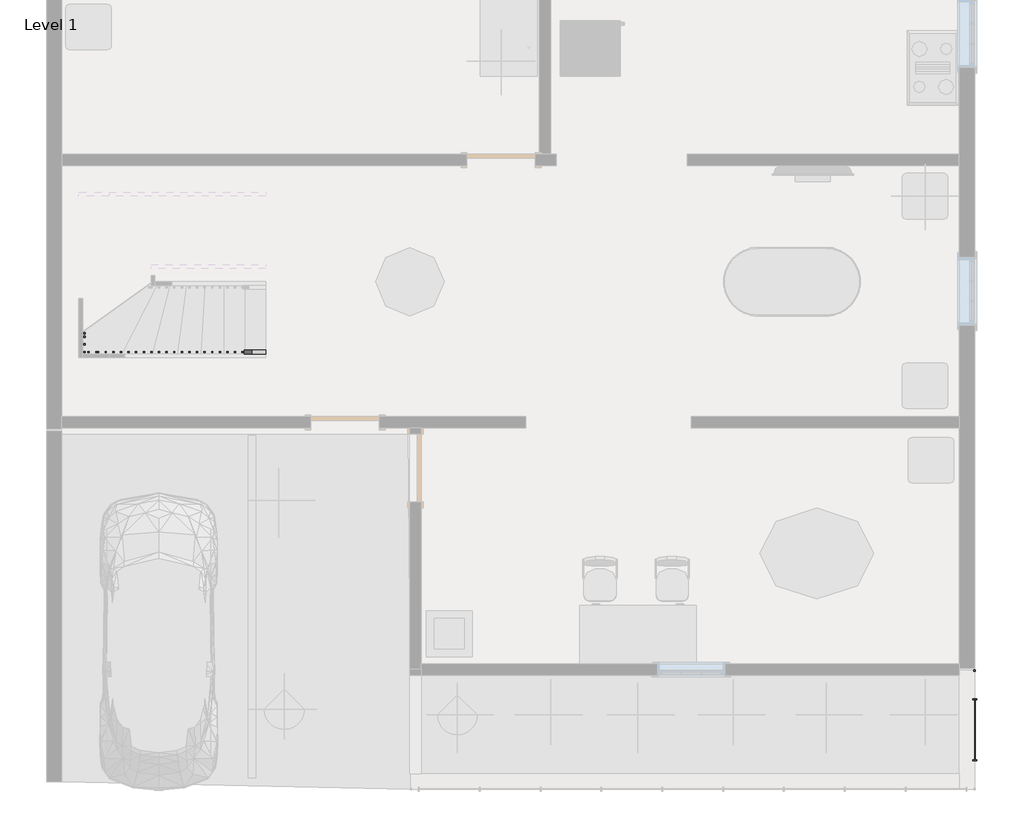
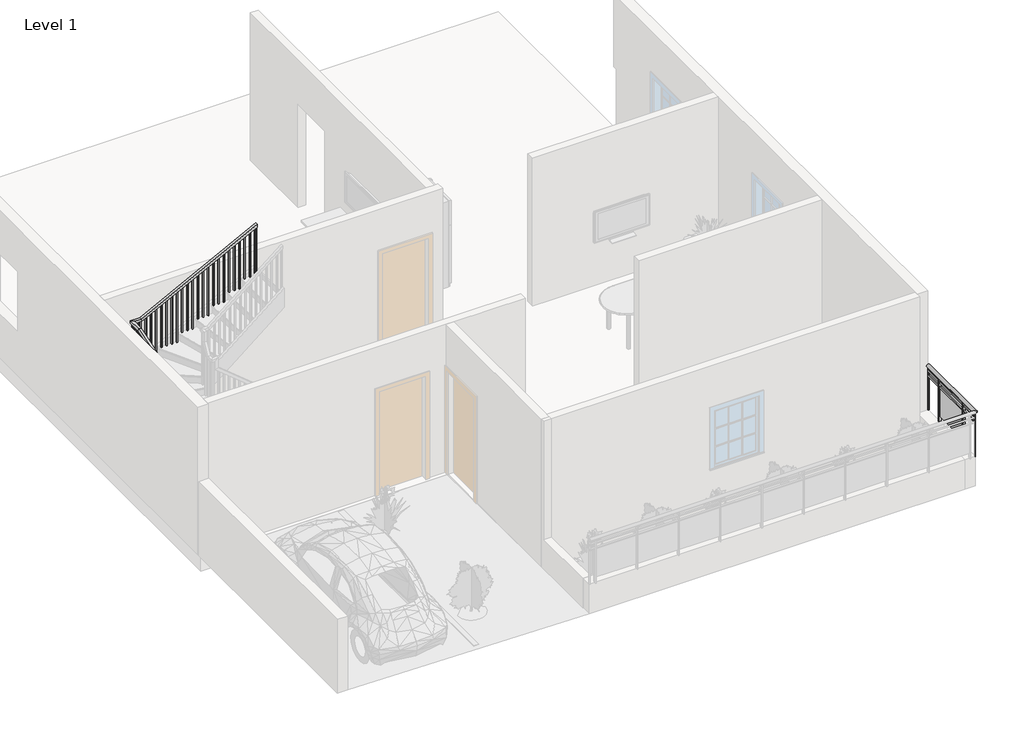
# One storey, part 2 of 3: 2 railings.
"""IFC4 building model written with IfcOpenShell, lengths in millimetres."""

from ifc_helpers import new_model, si_unit, point, frame, origin, place, context, project, spatial, polyline, ellipse_curve, trimmed, outline, extrude, faceted_brep, element, save
from ifc_brep_helpers import plane_surface, extruded_surface, advanced_brep

model = new_model("IFC4")

# Units and contexts
model_context = context("Model", 3, world=origin())
ifc_project = project(units=[si_unit("LENGTHUNIT", "METRE", prefix="MILLI")], contexts=[model_context])

# Site, building, storey
site = spatial("IfcSite", under=ifc_project)
building = spatial("IfcBuilding", under=site)
storey = spatial("IfcBuildingStorey", under=building, Name="Level 1", Elevation=0.0)

# Railings
placement = place(None, origin())
element("IfcRailing", 1, ObjectType="Glass Panel - Bottom Fill", at=placement, inside=storey, context=model_context, shape_type="SolidModel", body=[
    advanced_brep(
    [(-291.5234692, -2386.0883114, 1524.0), (-367.7234692, -2386.0883114, 1524.0), (-291.5234692, -3973.5883114, 1524.0), (-367.7234692, -3973.5883114, 1524.0)],
    [
        (0, 1, ellipse_curve(frame((-329.6234692, -2386.0883114, 1524.0), z_axis=(0.0, 1.0, 0.0), x_axis=(-1.0, 0.0, 0.0)), 38.1, 28.575)),
        (1, 0, ellipse_curve(frame((-329.6234692, -2386.0883114, 1524.0), z_axis=(0.0, 1.0, 0.0), x_axis=(-1.0, 0.0, 0.0)), 38.1, 28.575)),
        (2, 3, ellipse_curve(frame((-329.6234692, -3973.5883114, 1524.0), z_axis=(0.0, -1.0, 0.0), x_axis=(-1.0, 0.0, 0.0)), 38.1, 28.575)),
        (3, 2, ellipse_curve(frame((-329.6234692, -3973.5883114, 1524.0), z_axis=(0.0, -1.0, 0.0), x_axis=(-1.0, 0.0, 0.0)), 38.1, 28.575)),
        (0, 2),
        (3, 1),
    ],
    [
        plane_surface(frame((-329.6234692, -2386.0883114, 1524.0), z_axis=(0.0, 1.0, 0.0), x_axis=(0.0, 0.0, -1.0))),
        plane_surface(frame((-329.6234692, -3973.5883114, 1524.0), z_axis=(0.0, -1.0, 0.0), x_axis=(0.0, 0.0, -1.0))),
        extruded_surface(trimmed(ellipse_curve(frame((-329.6234692, -3973.5883114, 1524.0), z_axis=(0.0, 1.0, 0.0), x_axis=(-1.0, 0.0, 0.0)), 38.1, 28.575), [point((-291.5234692, -3973.5883114, 1524.0))], [point((-367.7234692, -3973.5883114, 1524.0))], True, "CARTESIAN"), (0.0, 1587.5, 0.0), 1587.5),
        extruded_surface(trimmed(ellipse_curve(frame((-329.6234692, -3973.5883114, 1524.0), z_axis=(0.0, 1.0, 0.0), x_axis=(-1.0, 0.0, 0.0)), 38.1, 28.575), [point((-367.7234692, -3973.5883114, 1524.0))], [point((-291.5234692, -3973.5883114, 1524.0))], True, "CARTESIAN"), (0.0, 1587.5, 0.0), 1587.5),
    ],
    [
        (0, [[1, 2]]),
        (1, [[3, 4]]),
        (2, [[-1, 5, -4, 6]]),
        (3, [[-2, -6, -3, -5]]),
    ],
),
    extrude(outline(polyline([(-342.3234692, -2386.0883114), (-316.9234692, -2386.0883114), (-316.9234692, -3973.5883114), (-342.3234692, -3973.5883114), (-342.3234692, -2386.0883114)])), frame((0.0, 0.0, 1409.7), z_axis=(0.0, 0.0, 1.0), x_axis=(1.0, 0.0, 0.0)), (0.0, 0.0, 1.0), 25.4),
    extrude(outline(polyline([(-342.3234692, -2386.0883114), (-316.9234692, -2386.0883114), (-316.9234692, -3973.5883114), (-342.3234692, -3973.5883114), (-342.3234692, -2386.0883114)])), frame((0.0, 0.0, 1308.1), z_axis=(0.0, 0.0, 1.0), x_axis=(1.0, 0.0, 0.0)), (0.0, 0.0, 1.0), 25.4),
    extrude(outline(polyline([(-355.0234692, -3579.8883114), (-304.2234692, -3579.8883114), (-304.2234692, -3592.5883114), (-355.0234692, -3592.5883114), (-355.0234692, -3579.8883114)])), frame((0.0, 0.0, 609.6), z_axis=(0.0, 0.0, 1.0), x_axis=(1.0, 0.0, 0.0)), (0.0, 0.0, 1.0), 885.6788223),
    extrude(outline(polyline([(-323.0883121, -2773.4383114), (-323.0883121, -3586.2383114), (-329.4383121, -3586.2383114), (-329.4383121, -2773.4383114), (-323.0883121, -2773.4383114)])), frame((0.0, 0.0, 711.2), z_axis=(0.0, 0.0, 1.0), x_axis=(1.0, 0.0, 0.0)), (0.0, 0.0, 1.0), 596.9),
    extrude(outline(polyline([(-355.0234692, -2767.0883114), (-304.2234692, -2767.0883114), (-304.2234692, -2779.7883114), (-355.0234692, -2779.7883114), (-355.0234692, -2767.0883114)])), frame((0.0, 0.0, 609.6), z_axis=(0.0, 0.0, 1.0), x_axis=(1.0, 0.0, 0.0)), (0.0, 0.0, 1.0), 885.6788223),
    extrude(outline(polyline([(-339.1484692, -3960.8883114), (-320.0984692, -3960.8883114), (-320.0984692, -3979.9383114), (-339.1484692, -3979.9383114), (-339.1484692, -3960.8883114)])), frame((0.0, 0.0, 609.6), z_axis=(0.0, 0.0, 1.0), x_axis=(1.0, 0.0, 0.0)), (0.0, 0.0, 1.0), 885.6788223),
    extrude(outline(polyline([(-339.1484692, -2379.7383114), (-320.0984692, -2379.7383114), (-320.0984692, -2398.7883114), (-339.1484692, -2398.7883114), (-339.1484692, -2379.7383114)])), frame((0.0, 0.0, 609.6), z_axis=(0.0, 0.0, 1.0), x_axis=(1.0, 0.0, 0.0)), (0.0, 0.0, 1.0), 885.6788223),
])
element("IfcRailing", 2, ObjectType="Handrail - Rectangular", at=placement, inside=storey, context=model_context, shape_type="SolidModel", body=[
    faceted_brep([(-9800.0917773, 1843.0116886, 1109.0771751), (-9800.0917773, 1843.0116886, 1051.9280057), (-9800.0917773, 1893.8116886, 1051.9280057), (-9800.0917773, 1893.8116886, 1109.0771751), (-12060.0736338, 1843.0116886, 2273.7644996), (-12072.3936851, 1843.0116886, 2222.9644996), (-12072.3936851, 1893.8116886, 2222.9644996), (-12060.0736338, 1893.8116886, 2273.7644996), (-12242.2234692, 1843.0116886, 2273.7644996), (-12242.2234692, 1843.0116886, 2222.9644996), (-12191.4234692, 1893.8116886, 2222.9644996), (-12191.4234692, 1893.8116886, 2273.7644996), (-12242.2234692, 2120.1656412, 2273.7644996), (-12242.2234692, 2128.1162174, 2222.9644996), (-12191.4234692, 2128.1162174, 2222.9644996), (-12191.4234692, 2120.1656412, 2273.7644996), (-12242.2234692, 3674.057736, 2772.3688337), (-12242.2234692, 3682.0083121, 2721.5688337), (-12191.4234692, 3682.0083121, 2721.5688337), (-12191.4234692, 3674.057736, 2772.3688337), (-12242.2234692, 3951.2116886, 2772.3688337), (-12242.2234692, 3951.2116886, 2721.5688337), (-12191.4234692, 3900.4116886, 2721.5688337), (-12191.4234692, 3900.4116886, 2772.3688337), (-12060.0736338, 3951.2116886, 2772.3688337), (-12047.7535825, 3951.2116886, 2721.5688337), (-12047.7535825, 3900.4116886, 2721.5688337), (-12060.0736338, 3900.4116886, 2772.3688337), (-9800.0917773, 3951.2116886, 3937.0561582), (-9800.0917773, 3900.4116886, 3937.0561582), (-9800.0917773, 3900.4116886, 3879.9069889), (-9800.0917773, 3951.2116886, 3879.9069889)], [[[0, 1, 2, 3]], [[1, 0, 4, 5]], [[2, 1, 5, 6]], [[3, 2, 6, 7]], [[0, 3, 7, 4]], [[5, 4, 8, 9]], [[6, 5, 9, 10]], [[7, 6, 10, 11]], [[4, 7, 11, 8]], [[9, 8, 12, 13]], [[10, 9, 13, 14]], [[11, 10, 14, 15]], [[8, 11, 15, 12]], [[13, 12, 16, 17]], [[14, 13, 17, 18]], [[15, 14, 18, 19]], [[12, 15, 19, 16]], [[17, 16, 20, 21]], [[18, 17, 21, 22]], [[19, 18, 22, 23]], [[16, 19, 23, 20]], [[21, 20, 24, 25]], [[22, 21, 25, 26]], [[23, 22, 26, 27]], [[20, 23, 27, 24]], [[28, 29, 30, 31]], [[25, 24, 28, 31]], [[26, 25, 31, 30]], [[27, 26, 30, 29]], [[24, 27, 29, 28]]]),
    extrude(outline(polyline([(3862.2268642, -9834.3986338), (2878.6666667, -9834.3986338), (2878.6666667, -9815.3486338), (3872.0443296, -9815.3486338), (3862.2268642, -9834.3986338)])), frame((0.0, 3916.2866886, 0.0), z_axis=(0.0, 1.0, 0.0), x_axis=(0.0, 0.0, 1.0)), (0.0, 0.0, 1.0), 19.05),
    extrude(outline(polyline([(3809.8670491, -9935.9986338), (2878.6666667, -9935.9986338), (2878.6666667, -9916.9486338), (3819.6845145, -9916.9486338), (3809.8670491, -9935.9986338)])), frame((0.0, 3916.2866886, 0.0), z_axis=(0.0, 1.0, 0.0), x_axis=(0.0, 0.0, 1.0)), (0.0, 0.0, 1.0), 19.05),
    extrude(outline(polyline([(3757.507234, -10037.5986338), (2878.6666667, -10037.5986338), (2878.6666667, -10018.5486338), (3767.3246993, -10018.5486338), (3757.507234, -10037.5986338)])), frame((0.0, 3916.2866886, 0.0), z_axis=(0.0, 1.0, 0.0), x_axis=(0.0, 0.0, 1.0)), (0.0, 0.0, 1.0), 19.05),
    extrude(outline(polyline([(3705.1474189, -10139.1986338), (2709.3333333, -10139.1986338), (2709.3333333, -10120.1486338), (3714.9648842, -10120.1486338), (3705.1474189, -10139.1986338)])), frame((0.0, 3916.2866886, 0.0), z_axis=(0.0, 1.0, 0.0), x_axis=(0.0, 0.0, 1.0)), (0.0, 0.0, 1.0), 19.05),
    extrude(outline(polyline([(3652.7876038, -10240.7986338), (2709.3333333, -10240.7986338), (2709.3333333, -10221.7486338), (3662.6050691, -10221.7486338), (3652.7876038, -10240.7986338)])), frame((0.0, 3916.2866886, 0.0), z_axis=(0.0, 1.0, 0.0), x_axis=(0.0, 0.0, 1.0)), (0.0, 0.0, 1.0), 19.05),
    extrude(outline(polyline([(3600.4277887, -10342.3986338), (2709.3333333, -10342.3986338), (2709.3333333, -10323.3486338), (3610.245254, -10323.3486338), (3600.4277887, -10342.3986338)])), frame((0.0, 3916.2866886, 0.0), z_axis=(0.0, 1.0, 0.0), x_axis=(0.0, 0.0, 1.0)), (0.0, 0.0, 1.0), 19.05),
    extrude(outline(polyline([(3548.0679735, -10443.9986338), (2540.0, -10443.9986338), (2540.0, -10424.9486338), (3557.8854389, -10424.9486338), (3548.0679735, -10443.9986338)])), frame((0.0, 3916.2866886, 0.0), z_axis=(0.0, 1.0, 0.0), x_axis=(0.0, 0.0, 1.0)), (0.0, 0.0, 1.0), 19.05),
    extrude(outline(polyline([(3495.7081584, -10545.5986338), (2540.0, -10545.5986338), (2540.0, -10526.5486338), (3505.5256238, -10526.5486338), (3495.7081584, -10545.5986338)])), frame((0.0, 3916.2866886, 0.0), z_axis=(0.0, 1.0, 0.0), x_axis=(0.0, 0.0, 1.0)), (0.0, 0.0, 1.0), 19.05),
    extrude(outline(polyline([(3443.3483433, -10647.1986338), (2540.0, -10647.1986338), (2540.0, -10628.1486338), (3453.1658086, -10628.1486338), (3443.3483433, -10647.1986338)])), frame((0.0, 3916.2866886, 0.0), z_axis=(0.0, 1.0, 0.0), x_axis=(0.0, 0.0, 1.0)), (0.0, 0.0, 1.0), 19.05),
    extrude(outline(polyline([(3390.9885282, -10748.7986338), (2370.6666667, -10748.7986338), (2370.6666667, -10729.7486338), (3400.8059935, -10729.7486338), (3390.9885282, -10748.7986338)])), frame((0.0, 3916.2866886, 0.0), z_axis=(0.0, 1.0, 0.0), x_axis=(0.0, 0.0, 1.0)), (0.0, 0.0, 1.0), 19.05),
    extrude(outline(polyline([(3338.6287131, -10850.3986338), (2370.6666667, -10850.3986338), (2370.6666667, -10831.3486338), (3348.4461784, -10831.3486338), (3338.6287131, -10850.3986338)])), frame((0.0, 3916.2866886, 0.0), z_axis=(0.0, 1.0, 0.0), x_axis=(0.0, 0.0, 1.0)), (0.0, 0.0, 1.0), 19.05),
    extrude(outline(polyline([(3286.268898, -10951.9986338), (2370.6666667, -10951.9986338), (2370.6666667, -10932.9486338), (3296.0863633, -10932.9486338), (3286.268898, -10951.9986338)])), frame((0.0, 3916.2866886, 0.0), z_axis=(0.0, 1.0, 0.0), x_axis=(0.0, 0.0, 1.0)), (0.0, 0.0, 1.0), 19.05),
    extrude(outline(polyline([(3233.9090828, -11053.5986338), (2201.3333333, -11053.5986338), (2201.3333333, -11034.5486338), (3243.7265482, -11034.5486338), (3233.9090828, -11053.5986338)])), frame((0.0, 3916.2866886, 0.0), z_axis=(0.0, 1.0, 0.0), x_axis=(0.0, 0.0, 1.0)), (0.0, 0.0, 1.0), 19.05),
    extrude(outline(polyline([(3181.5492677, -11155.1986338), (2201.3333333, -11155.1986338), (2201.3333333, -11136.1486338), (3191.3667331, -11136.1486338), (3181.5492677, -11155.1986338)])), frame((0.0, 3916.2866886, 0.0), z_axis=(0.0, 1.0, 0.0), x_axis=(0.0, 0.0, 1.0)), (0.0, 0.0, 1.0), 19.05),
    extrude(outline(polyline([(3129.1894526, -11256.7986338), (2201.3333333, -11256.7986338), (2201.3333333, -11237.7486338), (3139.0069179, -11237.7486338), (3129.1894526, -11256.7986338)])), frame((0.0, 3916.2866886, 0.0), z_axis=(0.0, 1.0, 0.0), x_axis=(0.0, 0.0, 1.0)), (0.0, 0.0, 1.0), 19.05),
    extrude(outline(polyline([(3076.8296375, -11358.3986338), (2032.0, -11358.3986338), (2032.0, -11339.3486338), (3086.6471028, -11339.3486338), (3076.8296375, -11358.3986338)])), frame((0.0, 3916.2866886, 0.0), z_axis=(0.0, 1.0, 0.0), x_axis=(0.0, 0.0, 1.0)), (0.0, 0.0, 1.0), 19.05),
    extrude(outline(polyline([(3024.4698224, -11459.9986338), (2032.0, -11459.9986338), (2032.0, -11440.9486338), (3034.2872877, -11440.9486338), (3024.4698224, -11459.9986338)])), frame((0.0, 3916.2866886, 0.0), z_axis=(0.0, 1.0, 0.0), x_axis=(0.0, 0.0, 1.0)), (0.0, 0.0, 1.0), 19.05),
    extrude(outline(polyline([(2972.1100073, -11561.5986338), (2032.0, -11561.5986338), (2032.0, -11542.5486338), (2981.9274726, -11542.5486338), (2972.1100073, -11561.5986338)])), frame((0.0, 3916.2866886, 0.0), z_axis=(0.0, 1.0, 0.0), x_axis=(0.0, 0.0, 1.0)), (0.0, 0.0, 1.0), 19.05),
    extrude(outline(polyline([(2919.7501921, -11663.1986338), (2032.0, -11663.1986338), (2032.0, -11644.1486338), (2929.5676575, -11644.1486338), (2919.7501921, -11663.1986338)])), frame((0.0, 3916.2866886, 0.0), z_axis=(0.0, 1.0, 0.0), x_axis=(0.0, 0.0, 1.0)), (0.0, 0.0, 1.0), 19.05),
    extrude(outline(polyline([(2867.390377, -11764.7986338), (1862.6666667, -11764.7986338), (1862.6666667, -11745.7486338), (2877.2078424, -11745.7486338), (2867.390377, -11764.7986338)])), frame((0.0, 3916.2866886, 0.0), z_axis=(0.0, 1.0, 0.0), x_axis=(0.0, 0.0, 1.0)), (0.0, 0.0, 1.0), 19.05),
    extrude(outline(polyline([(2815.0305619, -11866.3986338), (1862.6666667, -11866.3986338), (1862.6666667, -11847.3486338), (2824.8480272, -11847.3486338), (2815.0305619, -11866.3986338)])), frame((0.0, 3916.2866886, 0.0), z_axis=(0.0, 1.0, 0.0), x_axis=(0.0, 0.0, 1.0)), (0.0, 0.0, 1.0), 19.05),
    extrude(outline(polyline([(2762.6707468, -11967.9986338), (1862.6666667, -11967.9986338), (1862.6666667, -11948.9486338), (2772.4882121, -11948.9486338), (2762.6707468, -11967.9986338)])), frame((0.0, 3916.2866886, 0.0), z_axis=(0.0, 1.0, 0.0), x_axis=(0.0, 0.0, 1.0)), (0.0, 0.0, 1.0), 19.05),
    extrude(outline(polyline([(-12124.7484692, 3935.3366886), (-12105.6984692, 3935.3366886), (-12105.6984692, 3916.2866886), (-12124.7484692, 3916.2866886), (-12124.7484692, 3935.3366886)])), frame((0.0, 0.0, 1862.6666667), z_axis=(0.0, 0.0, 1.0), x_axis=(1.0, 0.0, 0.0)), (0.0, 0.0, 1.0), 858.902167),
    extrude(outline(polyline([(-12226.3484692, 3867.732736), (-12226.3484692, 3886.782736), (-12207.2984692, 3886.782736), (-12207.2984692, 3867.732736), (-12226.3484692, 3867.732736)])), frame((0.0, 0.0, 1862.6666667), z_axis=(0.0, 0.0, 1.0), x_axis=(1.0, 0.0, 0.0)), (0.0, 0.0, 1.0), 858.902167),
    extrude(outline(polyline([(-12226.3484692, 3766.132736), (-12226.3484692, 3785.182736), (-12207.2984692, 3785.182736), (-12207.2984692, 3766.132736), (-12226.3484692, 3766.132736)])), frame((0.0, 0.0, 1862.6666667), z_axis=(0.0, 0.0, 1.0), x_axis=(1.0, 0.0, 0.0)), (0.0, 0.0, 1.0), 858.902167),
    extrude(outline(polyline([(3653.6906412, 2712.4824155), (3653.6906412, 1693.3333333), (3634.6406412, 1693.3333333), (3634.6406412, 2706.3697564), (3653.6906412, 2712.4824155)])), frame((-12226.3484692, 0.0, 0.0), z_axis=(1.0, 0.0, 0.0), x_axis=(0.0, 1.0, 0.0)), (0.0, 0.0, 1.0), 19.05),
    extrude(outline(polyline([(3552.0906412, 2679.8815673), (3552.0906412, 1693.3333333), (3533.0406412, 1693.3333333), (3533.0406412, 2673.7689082), (3552.0906412, 2679.8815673)])), frame((-12226.3484692, 0.0, 0.0), z_axis=(1.0, 0.0, 0.0), x_axis=(0.0, 1.0, 0.0)), (0.0, 0.0, 1.0), 19.05),
    extrude(outline(polyline([(3450.4906412, 2647.280719), (3450.4906412, 1693.3333333), (3431.4406412, 1693.3333333), (3431.4406412, 2641.16806), (3450.4906412, 2647.280719)])), frame((-12226.3484692, 0.0, 0.0), z_axis=(1.0, 0.0, 0.0), x_axis=(0.0, 1.0, 0.0)), (0.0, 0.0, 1.0), 19.05),
    extrude(outline(polyline([(3348.8906412, 2614.6798708), (3348.8906412, 1693.3333333), (3329.8406412, 1693.3333333), (3329.8406412, 2608.5672118), (3348.8906412, 2614.6798708)])), frame((-12226.3484692, 0.0, 0.0), z_axis=(1.0, 0.0, 0.0), x_axis=(0.0, 1.0, 0.0)), (0.0, 0.0, 1.0), 19.05),
    extrude(outline(polyline([(3247.2906412, 2582.0790226), (3247.2906412, 1693.3333333), (3228.2406412, 1693.3333333), (3228.2406412, 2575.9663635), (3247.2906412, 2582.0790226)])), frame((-12226.3484692, 0.0, 0.0), z_axis=(1.0, 0.0, 0.0), x_axis=(0.0, 1.0, 0.0)), (0.0, 0.0, 1.0), 19.05),
    extrude(outline(polyline([(3145.6906412, 2549.4781744), (3145.6906412, 1693.3333333), (3126.6406412, 1693.3333333), (3126.6406412, 2543.3655153), (3145.6906412, 2549.4781744)])), frame((-12226.3484692, 0.0, 0.0), z_axis=(1.0, 0.0, 0.0), x_axis=(0.0, 1.0, 0.0)), (0.0, 0.0, 1.0), 19.05),
    extrude(outline(polyline([(3044.0906412, 2516.8773261), (3044.0906412, 1524.0), (3025.0406412, 1524.0), (3025.0406412, 2510.7646671), (3044.0906412, 2516.8773261)])), frame((-12226.3484692, 0.0, 0.0), z_axis=(1.0, 0.0, 0.0), x_axis=(0.0, 1.0, 0.0)), (0.0, 0.0, 1.0), 19.05),
    extrude(outline(polyline([(2942.4906412, 2484.2764779), (2942.4906412, 1524.0), (2923.4406412, 1524.0), (2923.4406412, 2478.1638189), (2942.4906412, 2484.2764779)])), frame((-12226.3484692, 0.0, 0.0), z_axis=(1.0, 0.0, 0.0), x_axis=(0.0, 1.0, 0.0)), (0.0, 0.0, 1.0), 19.05),
    extrude(outline(polyline([(2840.8906412, 2451.6756297), (2840.8906412, 1524.0), (2821.8406412, 1524.0), (2821.8406412, 2445.5629706), (2840.8906412, 2451.6756297)])), frame((-12226.3484692, 0.0, 0.0), z_axis=(1.0, 0.0, 0.0), x_axis=(0.0, 1.0, 0.0)), (0.0, 0.0, 1.0), 19.05),
    extrude(outline(polyline([(2739.2906412, 2419.0747814), (2739.2906412, 1524.0), (2720.2406412, 1524.0), (2720.2406412, 2412.9621224), (2739.2906412, 2419.0747814)])), frame((-12226.3484692, 0.0, 0.0), z_axis=(1.0, 0.0, 0.0), x_axis=(0.0, 1.0, 0.0)), (0.0, 0.0, 1.0), 19.05),
    extrude(outline(polyline([(2637.6906412, 2386.4739332), (2637.6906412, 1354.6666667), (2618.6406412, 1354.6666667), (2618.6406412, 2380.3612742), (2637.6906412, 2386.4739332)])), frame((-12226.3484692, 0.0, 0.0), z_axis=(1.0, 0.0, 0.0), x_axis=(0.0, 1.0, 0.0)), (0.0, 0.0, 1.0), 19.05),
    extrude(outline(polyline([(2536.0906412, 2353.873085), (2536.0906412, 1354.6666667), (2517.0406412, 1354.6666667), (2517.0406412, 2347.7604259), (2536.0906412, 2353.873085)])), frame((-12226.3484692, 0.0, 0.0), z_axis=(1.0, 0.0, 0.0), x_axis=(0.0, 1.0, 0.0)), (0.0, 0.0, 1.0), 19.05),
    extrude(outline(polyline([(2434.4906412, 2321.2722368), (2434.4906412, 1354.6666667), (2415.4406412, 1354.6666667), (2415.4406412, 2315.1595777), (2434.4906412, 2321.2722368)])), frame((-12226.3484692, 0.0, 0.0), z_axis=(1.0, 0.0, 0.0), x_axis=(0.0, 1.0, 0.0)), (0.0, 0.0, 1.0), 19.05),
    extrude(outline(polyline([(2332.8906412, 2288.6713885), (2332.8906412, 1354.6666667), (2313.8406412, 1354.6666667), (2313.8406412, 2282.5587295), (2332.8906412, 2288.6713885)])), frame((-12226.3484692, 0.0, 0.0), z_axis=(1.0, 0.0, 0.0), x_axis=(0.0, 1.0, 0.0)), (0.0, 0.0, 1.0), 19.05),
    extrude(outline(polyline([(2231.2906412, 2256.0705403), (2231.2906412, 1354.6666667), (2212.2406412, 1354.6666667), (2212.2406412, 2249.9578813), (2231.2906412, 2256.0705403)])), frame((-12226.3484692, 0.0, 0.0), z_axis=(1.0, 0.0, 0.0), x_axis=(0.0, 1.0, 0.0)), (0.0, 0.0, 1.0), 19.05),
    extrude(outline(polyline([(-12226.3484692, 2062.0866886), (-12226.3484692, 2081.1366886), (-12207.2984692, 2081.1366886), (-12207.2984692, 2062.0866886), (-12226.3484692, 2062.0866886)])), frame((0.0, 0.0, 1185.3333333), z_axis=(0.0, 0.0, 1.0), x_axis=(1.0, 0.0, 0.0)), (0.0, 0.0, 1.0), 1037.6311663),
    extrude(outline(polyline([(-12226.3484692, 1960.4866886), (-12226.3484692, 1979.5366886), (-12207.2984692, 1979.5366886), (-12207.2984692, 1960.4866886), (-12226.3484692, 1960.4866886)])), frame((0.0, 0.0, 1185.3333333), z_axis=(0.0, 0.0, 1.0), x_axis=(1.0, 0.0, 0.0)), (0.0, 0.0, 1.0), 1037.6311663),
    extrude(outline(polyline([(-12152.1486338, 1858.8866886), (-12171.1986338, 1858.8866886), (-12171.1986338, 1877.9366886), (-12152.1486338, 1877.9366886), (-12152.1486338, 1858.8866886)])), frame((0.0, 0.0, 1185.3333333), z_axis=(0.0, 0.0, 1.0), x_axis=(1.0, 0.0, 0.0)), (0.0, 0.0, 1.0), 1037.6311663),
    extrude(outline(polyline([(2208.752671, -12044.8167773), (1185.3333333, -12044.8167773), (1185.3333333, -12025.7667773), (2198.9352056, -12025.7667773), (2208.752671, -12044.8167773)])), frame((0.0, 1858.8866886, 0.0), z_axis=(0.0, 1.0, 0.0), x_axis=(0.0, 0.0, 1.0)), (0.0, 0.0, 1.0), 19.05),
    extrude(outline(polyline([(2156.3928558, -11943.2167773), (1185.3333333, -11943.2167773), (1185.3333333, -11924.1667773), (2146.5753905, -11924.1667773), (2156.3928558, -11943.2167773)])), frame((0.0, 1858.8866886, 0.0), z_axis=(0.0, 1.0, 0.0), x_axis=(0.0, 0.0, 1.0)), (0.0, 0.0, 1.0), 19.05),
    extrude(outline(polyline([(2104.0330407, -11841.6167773), (1185.3333333, -11841.6167773), (1185.3333333, -11822.5667773), (2094.2155754, -11822.5667773), (2104.0330407, -11841.6167773)])), frame((0.0, 1858.8866886, 0.0), z_axis=(0.0, 1.0, 0.0), x_axis=(0.0, 0.0, 1.0)), (0.0, 0.0, 1.0), 19.05),
    extrude(outline(polyline([(2051.6732256, -11740.0167773), (1185.3333333, -11740.0167773), (1185.3333333, -11720.9667773), (2041.8557603, -11720.9667773), (2051.6732256, -11740.0167773)])), frame((0.0, 1858.8866886, 0.0), z_axis=(0.0, 1.0, 0.0), x_axis=(0.0, 0.0, 1.0)), (0.0, 0.0, 1.0), 19.05),
    extrude(outline(polyline([(1999.3134105, -11638.4167773), (1016.0, -11638.4167773), (1016.0, -11619.3667773), (1989.4959452, -11619.3667773), (1999.3134105, -11638.4167773)])), frame((0.0, 1858.8866886, 0.0), z_axis=(0.0, 1.0, 0.0), x_axis=(0.0, 0.0, 1.0)), (0.0, 0.0, 1.0), 19.05),
    extrude(outline(polyline([(1946.9535954, -11536.8167773), (1016.0, -11536.8167773), (1016.0, -11517.7667773), (1937.13613, -11517.7667773), (1946.9535954, -11536.8167773)])), frame((0.0, 1858.8866886, 0.0), z_axis=(0.0, 1.0, 0.0), x_axis=(0.0, 0.0, 1.0)), (0.0, 0.0, 1.0), 19.05),
    extrude(outline(polyline([(1894.5937803, -11435.2167773), (1016.0, -11435.2167773), (1016.0, -11416.1667773), (1884.7763149, -11416.1667773), (1894.5937803, -11435.2167773)])), frame((0.0, 1858.8866886, 0.0), z_axis=(0.0, 1.0, 0.0), x_axis=(0.0, 0.0, 1.0)), (0.0, 0.0, 1.0), 19.05),
    extrude(outline(polyline([(1842.2339651, -11333.6167773), (1016.0, -11333.6167773), (1016.0, -11314.5667773), (1832.4164998, -11314.5667773), (1842.2339651, -11333.6167773)])), frame((0.0, 1858.8866886, 0.0), z_axis=(0.0, 1.0, 0.0), x_axis=(0.0, 0.0, 1.0)), (0.0, 0.0, 1.0), 19.05),
    extrude(outline(polyline([(1789.87415, -11232.0167773), (846.6666667, -11232.0167773), (846.6666667, -11212.9667773), (1780.0566847, -11212.9667773), (1789.87415, -11232.0167773)])), frame((0.0, 1858.8866886, 0.0), z_axis=(0.0, 1.0, 0.0), x_axis=(0.0, 0.0, 1.0)), (0.0, 0.0, 1.0), 19.05),
    extrude(outline(polyline([(1737.5143349, -11130.4167773), (846.6666667, -11130.4167773), (846.6666667, -11111.3667773), (1727.6968696, -11111.3667773), (1737.5143349, -11130.4167773)])), frame((0.0, 1858.8866886, 0.0), z_axis=(0.0, 1.0, 0.0), x_axis=(0.0, 0.0, 1.0)), (0.0, 0.0, 1.0), 19.05),
    extrude(outline(polyline([(1685.1545198, -11028.8167773), (846.6666667, -11028.8167773), (846.6666667, -11009.7667773), (1675.3370545, -11009.7667773), (1685.1545198, -11028.8167773)])), frame((0.0, 1858.8866886, 0.0), z_axis=(0.0, 1.0, 0.0), x_axis=(0.0, 0.0, 1.0)), (0.0, 0.0, 1.0), 19.05),
    extrude(outline(polyline([(1632.7947047, -10927.2167773), (677.3333333, -10927.2167773), (677.3333333, -10908.1667773), (1622.9772393, -10908.1667773), (1632.7947047, -10927.2167773)])), frame((0.0, 1858.8866886, 0.0), z_axis=(0.0, 1.0, 0.0), x_axis=(0.0, 0.0, 1.0)), (0.0, 0.0, 1.0), 19.05),
    extrude(outline(polyline([(1580.4348896, -10825.6167773), (677.3333333, -10825.6167773), (677.3333333, -10806.5667773), (1570.6174242, -10806.5667773), (1580.4348896, -10825.6167773)])), frame((0.0, 1858.8866886, 0.0), z_axis=(0.0, 1.0, 0.0), x_axis=(0.0, 0.0, 1.0)), (0.0, 0.0, 1.0), 19.05),
    extrude(outline(polyline([(1528.0750744, -10724.0167773), (677.3333333, -10724.0167773), (677.3333333, -10704.9667773), (1518.2576091, -10704.9667773), (1528.0750744, -10724.0167773)])), frame((0.0, 1858.8866886, 0.0), z_axis=(0.0, 1.0, 0.0), x_axis=(0.0, 0.0, 1.0)), (0.0, 0.0, 1.0), 19.05),
    extrude(outline(polyline([(1475.7152593, -10622.4167773), (508.0, -10622.4167773), (508.0, -10603.3667773), (1465.897794, -10603.3667773), (1475.7152593, -10622.4167773)])), frame((0.0, 1858.8866886, 0.0), z_axis=(0.0, 1.0, 0.0), x_axis=(0.0, 0.0, 1.0)), (0.0, 0.0, 1.0), 19.05),
    extrude(outline(polyline([(1423.3554442, -10520.8167773), (508.0, -10520.8167773), (508.0, -10501.7667773), (1413.5379789, -10501.7667773), (1423.3554442, -10520.8167773)])), frame((0.0, 1858.8866886, 0.0), z_axis=(0.0, 1.0, 0.0), x_axis=(0.0, 0.0, 1.0)), (0.0, 0.0, 1.0), 19.05),
    extrude(outline(polyline([(1370.9956291, -10419.2167773), (508.0, -10419.2167773), (508.0, -10400.1667773), (1361.1781638, -10400.1667773), (1370.9956291, -10419.2167773)])), frame((0.0, 1858.8866886, 0.0), z_axis=(0.0, 1.0, 0.0), x_axis=(0.0, 0.0, 1.0)), (0.0, 0.0, 1.0), 19.05),
    extrude(outline(polyline([(1318.635814, -10317.6167773), (338.6666667, -10317.6167773), (338.6666667, -10298.5667773), (1308.8183486, -10298.5667773), (1318.635814, -10317.6167773)])), frame((0.0, 1858.8866886, 0.0), z_axis=(0.0, 1.0, 0.0), x_axis=(0.0, 0.0, 1.0)), (0.0, 0.0, 1.0), 19.05),
    extrude(outline(polyline([(1266.2759989, -10216.0167773), (338.6666667, -10216.0167773), (338.6666667, -10196.9667773), (1256.4585335, -10196.9667773), (1266.2759989, -10216.0167773)])), frame((0.0, 1858.8866886, 0.0), z_axis=(0.0, 1.0, 0.0), x_axis=(0.0, 0.0, 1.0)), (0.0, 0.0, 1.0), 19.05),
    extrude(outline(polyline([(1213.9161837, -10114.4167773), (338.6666667, -10114.4167773), (338.6666667, -10095.3667773), (1204.0987184, -10095.3667773), (1213.9161837, -10114.4167773)])), frame((0.0, 1858.8866886, 0.0), z_axis=(0.0, 1.0, 0.0), x_axis=(0.0, 0.0, 1.0)), (0.0, 0.0, 1.0), 19.05),
    extrude(outline(polyline([(1161.5563686, -10012.8167773), (169.3333333, -10012.8167773), (169.3333333, -9993.7667773), (1151.7389033, -9993.7667773), (1161.5563686, -10012.8167773)])), frame((0.0, 1858.8866886, 0.0), z_axis=(0.0, 1.0, 0.0), x_axis=(0.0, 0.0, 1.0)), (0.0, 0.0, 1.0), 19.05),
    extrude(outline(polyline([(1109.1965535, -9911.2167773), (169.3333333, -9911.2167773), (169.3333333, -9892.1667773), (1099.3790882, -9892.1667773), (1109.1965535, -9911.2167773)])), frame((0.0, 1858.8866886, 0.0), z_axis=(0.0, 1.0, 0.0), x_axis=(0.0, 0.0, 1.0)), (0.0, 0.0, 1.0), 19.05),
    extrude(outline(polyline([(-12069.5986338, 3935.3366886), (-12050.5486338, 3935.3366886), (-12050.5486338, 3916.2866886), (-12069.5986338, 3916.2866886), (-12069.5986338, 3935.3366886)])), frame((0.0, 0.0, 1862.6666667), z_axis=(0.0, 0.0, 1.0), x_axis=(1.0, 0.0, 0.0)), (0.0, 0.0, 1.0), 858.902167),
    extrude(outline(polyline([(-12226.3484692, 3916.2866886), (-12226.3484692, 3935.3366886), (-12207.2984692, 3935.3366886), (-12207.2984692, 3916.2866886), (-12226.3484692, 3916.2866886)])), frame((0.0, 0.0, 1862.6666667), z_axis=(0.0, 0.0, 1.0), x_axis=(1.0, 0.0, 0.0)), (0.0, 0.0, 1.0), 858.902167),
    extrude(outline(polyline([(3683.582736, 2722.0740262), (3683.582736, 1862.6666667), (3664.532736, 1862.6666667), (3664.532736, 2715.9613671), (3683.582736, 2722.0740262)])), frame((-12226.3484692, 0.0, 0.0), z_axis=(1.0, 0.0, 0.0), x_axis=(0.0, 1.0, 0.0)), (0.0, 0.0, 1.0), 19.05),
    extrude(outline(polyline([(-12226.3484692, 2110.6406412), (-12226.3484692, 2129.6906412), (-12207.2984692, 2129.6906412), (-12207.2984692, 2110.6406412), (-12226.3484692, 2110.6406412)])), frame((0.0, 0.0, 1185.3333333), z_axis=(0.0, 0.0, 1.0), x_axis=(1.0, 0.0, 0.0)), (0.0, 0.0, 1.0), 1037.6311663),
    extrude(outline(polyline([(-12207.2984692, 1858.8866886), (-12226.3484692, 1858.8866886), (-12226.3484692, 1877.9366886), (-12207.2984692, 1877.9366886), (-12207.2984692, 1858.8866886)])), frame((0.0, 0.0, 1185.3333333), z_axis=(0.0, 0.0, 1.0), x_axis=(1.0, 0.0, 0.0)), (0.0, 0.0, 1.0), 1037.6311663),
    extrude(outline(polyline([(2221.5240629, -12069.5986338), (1185.3333333, -12069.5986338), (1185.3333333, -12050.5486338), (2211.7065976, -12050.5486338), (2221.5240629, -12069.5986338)])), frame((0.0, 1858.8866886, 0.0), z_axis=(0.0, 1.0, 0.0), x_axis=(0.0, 0.0, 1.0)), (0.0, 0.0, 1.0), 19.05),
    extrude(outline(polyline([(3870.0895235, -9819.1417773), (2878.6666667, -9819.1417773), (2878.6666667, -9800.0917773), (3879.9069889, -9800.0917773), (3870.0895235, -9819.1417773)])), frame((0.0, 3916.2866886, 0.0), z_axis=(0.0, 1.0, 0.0), x_axis=(0.0, 0.0, 1.0)), (0.0, 0.0, 1.0), 19.05),
    extrude(outline(polyline([(1061.7454711, -9819.1417773), (169.3333333, -9819.1417773), (169.3333333, -9800.0917773), (1051.9280057, -9800.0917773), (1061.7454711, -9819.1417773)])), frame((0.0, 1858.8866886, 0.0), z_axis=(0.0, 1.0, 0.0), x_axis=(0.0, 0.0, 1.0)), (0.0, 0.0, 1.0), 19.05),
])

save(model, "model.ifc")

# Revit data of these elements
# Type "Glass Panel - Bottom Fill"
#   Assembly Code = "C2010400"
#   built-in parameter 1008612 = 0.0416667 (stored number, unit not read)
#   built-in parameter 1008611 = 0.0416667 (stored number, unit not read)
#   built-in parameter 1008609 = 0.333333 (stored number, unit not read)
#   built-in parameter 1008604 = 0.166667 (stored number, unit not read)
#   built-in parameter 1008603 = 0.166667 (stored number, unit not read)
#   Railing Height = 3' - 0"
#   built-in parameter 1008630 = 2
#   built-in parameter 1008610 = 2
#   built-in parameter 1008618 = Baluster - Square : 3/4"
# Type "Handrail - Rectangular"
#   Assembly Code = "C2010400"
#   built-in parameter 1008612 = 0.0416667 (stored number, unit not read)
#   built-in parameter 1008611 = 0.0416667 (stored number, unit not read)
#   built-in parameter 1008609 = 0.333333 (stored number, unit not read)
#   built-in parameter 1008604 = 0.166667 (stored number, unit not read)
#   built-in parameter 1008603 = 0.166667 (stored number, unit not read)
#   Railing Height = 3' - 0"
#   built-in parameter 1008630 = 2
#   built-in parameter 1008610 = 2
#   built-in parameter 1008618 = Baluster - Square : 3/4"
# Element 1 (IfcRailing, "Glass Panel - Bottom Fill")
#   built-in parameter 1008621 = 2 (stored number, unit not read)
#   Phase Created = New Construction
#   Materials on its faces: "Glass"
# Element 2 (IfcRailing, "Handrail - Rectangular")
#   Phase Created = New Construction
# Materials
#   "Glass": class "Glass", colour RGB 0 128 192, transparency 0.75, Description = "Soda Lime Glass", Cost = 0
